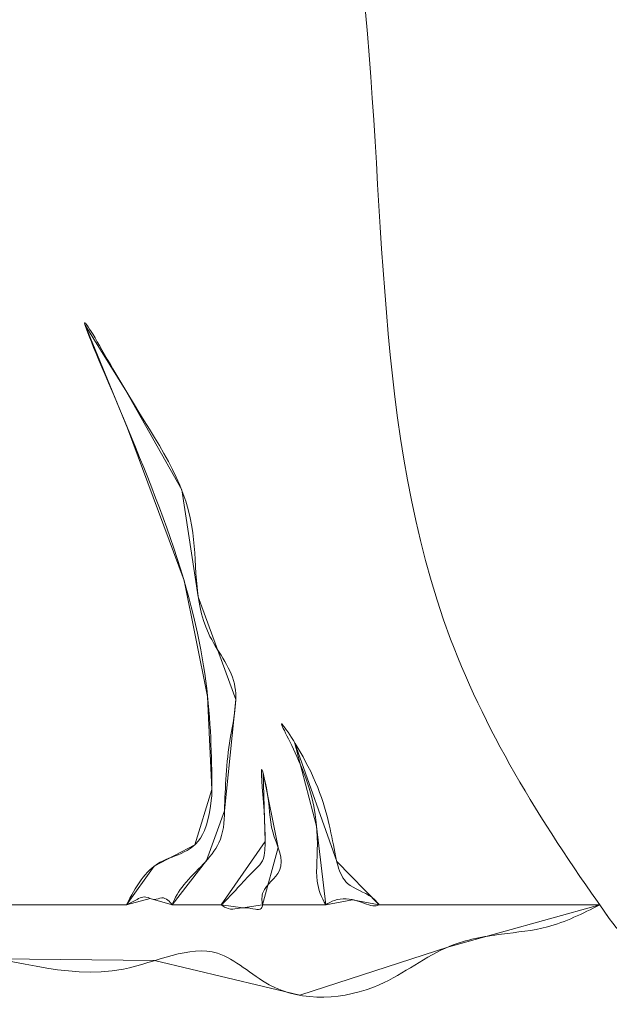
# Model space of a CAD drawing. Units: inches. Extents: x 2083 to 3317, y 1141 to 2115.
# Tile 6 of 256: x 2260 to 2278, y 1296 to 1327. Entities that reach past the tile are written whole.
import ezdxf

# ---------------------------------------------------------------- set-up
doc = ezdxf.new("R2010")
doc.units = ezdxf.units.IN
doc.layers.add('A-FURN', color=8, linetype='Continuous', lineweight=18)
doc.layers.add('www.cadblocksfree.com', color=7, linetype='Continuous', lineweight=9)
doc.layers.add('A-WALL-PATT', color=251, linetype='Continuous', lineweight=13, true_color=0x636466)

# ---------------------------------------------------------------- blocks, each defined once
blk = doc.blocks.new('bed')
at = {"layer": 'www.cadblocksfree.com', "ltscale": 0.2}
for points in [[(3426.379, 1449.413), (3426.379, 1470.154), (3363.387, 1470.154), (3363.387, 1447.076)], [(3363.387, 1445.539), (3363.387, 1443.892)], [(3363.387, 1442.495), (3363.387, 1440.369)], [(3363.387, 1438.564), (3363.387, 1431.137)]]:
    blk.add_lwpolyline(points, dxfattribs=at)
for points, knots in [([(3360.883, 1467.22), (3361.272, 1466.08), (3362.328, 1462.983), (3360.73, 1458.154), (3362.389, 1452.621), (3360.35, 1448.139), (3362.429, 1444.241), (3360.039, 1441.931), (3360.256, 1438.678), (3362.05, 1436.545), (3362.42, 1434.517), (3362.566, 1432.758), (3363.096, 1431.712), (3363.387, 1431.137)], [0, 0, 0, 0, 3.550403, 9.643115, 14.356056, 20.206026, 23.427697, 25.46537, 29.172767, 31.884544, 33.668442, 35.237641, 37.145618, 37.145618, 37.145618, 37.145618]), ([(3367.269, 1444.201), (3369.575, 1444.23), (3373.917, 1444.284), (3385.471, 1449.8), (3379.558, 1446.493), (3376.808, 1444.477), (3372.948, 1444.924), (3370.926, 1443.14), (3368.771, 1443.702), (3367.359, 1443.752), (3366.554, 1443.781)], [0, 0, 0, 0, 8.61026, 16.221274, 18.843057, 23.804898, 27.440828, 29.356102, 31.203478, 33.650687, 33.650687, 33.650687, 33.650687]), ([(3363.387, 1447.076), (3363.429, 1446.99), (3363.529, 1446.784), (3363.731, 1446.461), (3363.506, 1446.154), (3363.665, 1445.905), (3363.559, 1445.673), (3363.444, 1445.584), (3363.387, 1445.539)], [0, 0, 0, 0, 0.293454, 0.701471, 1.003873, 1.254893, 1.47342, 1.69185, 1.69185, 1.69185, 1.69185]), ([(3363.387, 1447.076), (3363.991, 1446.782), (3365.084, 1446.124), (3365.119, 1444.371), (3367.129, 1444.191), (3367.269, 1444.201)], [0.0122268, 0.0122268, 0.0122268, 0.0122268, 0.0594721, 0.1062177, 0.134458, 0.134458, 0.134458, 0.134458]), ([(3366.554, 1443.781), (3366.17, 1443.775), (3365.174, 1443.901), (3364.4, 1444.957), (3363.626, 1445.461), (3363.387, 1445.539)], [0.15648839, 0.15648839, 0.15648839, 0.15648839, 0.18439755, 0.23137648, 0.25059846, 0.25059846, 0.25059846, 0.25059846]), ([(3363.387, 1443.892), (3363.335, 1443.815), (3363.165, 1443.56), (3363.346, 1443.124), (3363.233, 1442.791), (3363.225, 1442.533), (3363.341, 1442.506), (3363.387, 1442.495)], [0, 0, 0, 0, 0.27176, 0.887321, 1.189132, 1.388142, 1.515331, 1.515331, 1.515331, 1.515331]), ([(3363.387, 1443.892), (3363.631, 1443.61), (3364.671, 1442.733), (3364.886, 1442.149), (3369.073, 1442.744), (3366.773, 1442.243), (3365.832, 1442.298), (3364.615, 1441.552), (3363.961, 1442.542), (3363.537, 1442.524), (3363.387, 1442.495)], [0.0595743, 0.0595743, 0.0595743, 0.0595743, 0.0807529, 0.1037415, 0.1697201, 0.1760361, 0.2071372, 0.2404744, 0.2623409, 0.2736605, 0.2736605, 0.2736605, 0.2736605]), ([(3362.928, 1430.813), (3365.944, 1432.958), (3375.455, 1438.993), (3392.12, 1438.03), (3404.249, 1440.73), (3408.408, 1442.961)], [0.102872, 0.102872, 0.102872, 0.102872, 0.37972, 0.957702, 1.313793, 1.313793, 1.313793, 1.313793]), ([(3363.387, 1440.369), (3363.634, 1440.51), (3364.527, 1440.899), (3366.485, 1440.246), (3370.203, 1442.295), (3367.731, 1440.636), (3365.42, 1440.07), (3364.035, 1439.913), (3363.795, 1438.935), (3363.482, 1438.64), (3363.387, 1438.564)], [0.013856, 0.013856, 0.013856, 0.013856, 0.0348738, 0.0888667, 0.1078792, 0.1267378, 0.158714, 0.1937575, 0.2174868, 0.2267221, 0.2267221, 0.2267221, 0.2267221]), ([(3363.387, 1440.369), (3363.445, 1440.274), (3363.571, 1440.065), (3363.607, 1439.678), (3363.531, 1439.31), (3363.405, 1439.003), (3363.329, 1438.751), (3363.372, 1438.611), (3363.387, 1438.564)], [0, 0, 0, 0, 0.329977, 0.725302, 1.129072, 1.442831, 1.734218, 1.878348, 1.878348, 1.878348, 1.878348])]:
    blk.add_open_spline(points, degree=3, knots=knots, dxfattribs=at)

msp = doc.modelspace()

# ---------------------------------------------------------------- hatches: boundary and pattern name
at = {"layer": 'A-WALL-PATT'}
h = msp.add_hatch(color=256, dxfattribs=at)
h.dxf.hatch_style = 1
h.paths.add_polyline_path([(3126.96, 2020.761), (2748.96, 2020.761), (2604.96, 2020.761), (2226.96, 2020.761), (2226.96, 1702.761), (2466.96, 1702.761), (2466.96, 1582.761), (2418.96, 1582.761), (2418.96, 1477.761), (2226.96, 1477.761), (2226.96, 1263.261), (2544.96, 1263.261), (2544.96, 1411.761), (2604.96, 1411.761), (2685.96, 1411.761), (2685.96, 1420.761), (2604.96, 1420.761), (2604.96, 1573.761), (2604.96, 1702.761), (2604.96, 2011.761), (2748.96, 2011.761), (2748.96, 1702.761), (2862.96, 1702.761), (2862.96, 1621.761), (2871.96, 1621.761), (2871.96, 1702.761), (2883.96, 1702.761), (2883.96, 1706.939, -0.026459), (2883.96, 1711.761), (2757.96, 1711.761), (2757.96, 1807.761), (2787.96, 1807.761), (2787.96, 1812.261), (2757.96, 1812.261), (2757.96, 2011.761), (2877.96, 2011.761), (2877.96, 1812.261), (2847.96, 1812.261), (2847.96, 1807.761), (2889.836, 1807.761), (2889.836, 1812.261), (2882.46, 1812.261), (2882.46, 2011.761), (3117.96, 2011.761), (3117.96, 1812.261), (2937.836, 1812.261), (2937.836, 1807.761), (2995.71, 1807.761), (2995.71, 1796.118), (3000.21, 1796.118), (3000.21, 1807.761), (3117.96, 1807.761), (3117.96, 1711.761), (3000.21, 1711.761), (3000.21, 1760.118), (2998.573, 1760.118, -0.020711), (2995.71, 1760.118), (2995.71, 1711.761), (2931.96, 1711.761), (2931.96, 1702.761), (3126.96, 1702.761)])
h.paths.add_polyline_path([(2471.46, 2011.761), (2471.46, 1810.011), (2462.717, 1810.011), (2462.717, 1805.511), (2505.96, 1805.511), (2505.96, 1810.011), (2475.96, 1810.011), (2475.96, 2011.761), (2595.96, 2011.761), (2595.96, 1810.011), (2565.96, 1810.011), (2565.96, 1805.511), (2595.96, 1805.511), (2595.96, 1711.761), (2235.96, 1711.761), (2235.96, 1805.511), (2353.71, 1805.511), (2353.71, 1796.054), (2358.21, 1796.054), (2358.21, 1805.511), (2414.717, 1805.511), (2414.717, 1810.011), (2235.96, 1810.011), (2235.96, 2011.761)], flags=16)
h.paths.add_polyline_path([(2270.205, 1994.61), (2270.205, 1970.61), (2246.205, 1970.61), (2246.205, 1994.61)], flags=0)
edge = h.paths.add_edge_path(flags=0)
edge.add_ellipse((2332.027, 1899.798), major_axis=(-3.043, 3.043), ratio=0.168252, start_angle=-161.3322, end_angle=-156.3071, ccw=False)
edge.add_ellipse((2333.082, 1898.744), major_axis=(-1.055, 1.055), ratio=0.453532, start_angle=-123.371, end_angle=-94.1591)
edge = h.paths.add_edge_path(flags=0)
edge.add_ellipse((2332.027, 1968.876), major_axis=(3.043, 3.043), ratio=0.168252, start_angle=18.6678, end_angle=23.6929)
edge.add_spline(control_points=[(2332.926, 1970.691), (2332.227, 1970.336), (2330.894, 1969.659), (2328.413, 1970.932), (2327.204, 1967.749), (2324.71, 1969.956), (2322.533, 1967.012), (2320.013, 1971.296), (2317.68, 1968.158), (2316.041, 1967.102), (2315.427, 1966.81)], knot_values=[0, 0, 0, 0, 2.267059, 4.324559, 6.685584, 8.878641, 11.121502, 14.300359, 17.755284, 19.732645, 19.732645, 19.732645, 19.732645], degree=3, periodic=0)
edge.add_ellipse((2332.027, 1968.876), major_axis=(3.043, 3.043), ratio=0.168252, start_angle=18.6678, end_angle=23.6929, ccw=False)
edge.add_ellipse((2333.082, 1969.931), major_axis=(1.055, 1.055), ratio=0.453532, start_angle=56.629, end_angle=85.8409, ccw=False)
edge = h.paths.add_edge_path(flags=0)
edge.add_spline(control_points=[(2296.428, 1967.988), (2293.628, 1965.336), (2287.704, 1959.727), (2299.744, 1949.996), (2294.533, 1935.669), (2290.573, 1920.604), (2293.394, 1909.974), (2296.185, 1904.967)], knot_values=[0.099185, 0.099185, 0.099185, 0.099185, 0.345301, 0.619822, 0.982653, 1.386093, 1.810555, 1.810555, 1.810555, 1.810555], degree=3, periodic=0)
edge.add_spline(control_points=[(2296.185, 1904.967), (2297.384, 1902.619), (2298.001, 1901.949), (2298.553, 1901.468)], knot_values=[0.006246, 0.006246, 0.006246, 0.006246, 0.055476, 0.055476, 0.055476, 0.055476], degree=3, periodic=0)
edge.add_spline(control_points=[(2298.553, 1901.468), (2297.259, 1900.923), (2295.225, 1900.232), (2293.06, 1900.614), (2292.101, 1900.788), (2292.09, 1900.791)], knot_values=[0.312835, 0.312835, 0.312835, 0.312835, 0.40178, 0.474987, 0.475903, 0.475903, 0.475903, 0.475903], degree=3, periodic=0)
edge.add_arc((2292.794, 1904.664), 3.937, 215.4209, 259.6982, ccw=False)
edge.add_spline(control_points=[(2289.585, 1902.382), (2289.477, 1902.535), (2289.368, 1902.688), (2289.261, 1902.841)], knot_values=[0.102872, 0.102872, 0.102872, 0.102872, 0.116896, 0.116896, 0.116896, 0.116896], degree=3, periodic=0)
edge.add_spline(control_points=[(2289.261, 1902.841), (2288.687, 1902.55), (2287.64, 1902.02), (2285.881, 1901.874), (2283.853, 1901.504), (2281.72, 1899.711), (2278.467, 1899.493), (2276.157, 1901.883), (2272.259, 1899.804), (2267.778, 1901.843), (2262.244, 1900.184), (2257.415, 1901.782), (2254.318, 1900.726), (2253.178, 1900.337)], knot_values=[0, 0, 0, 0, 1.907977, 3.477176, 5.261074, 7.972851, 11.680248, 13.717921, 16.939592, 22.789562, 27.502503, 33.595215, 37.145618, 37.145618, 37.145618, 37.145618], degree=3, periodic=0)
edge.add_line((2253.178, 1900.337), (2250.244, 1902.841))
edge.add_line((2250.244, 1902.841), (2250.244, 1965.833))
edge.add_line((2250.244, 1965.833), (2253.178, 1968.337))
edge.add_spline(control_points=[(2253.178, 1968.337), (2254.318, 1967.948), (2257.415, 1966.892), (2262.244, 1968.49), (2267.778, 1966.831), (2271.527, 1968.537), (2273.876, 1967.828), (2274.207, 1967.728)], knot_values=[0, 0, 0, 0, 0.09018, 0.244935, 0.364644, 0.513233, 0.537855, 0.537855, 0.537855, 0.537855], degree=3, periodic=0)
edge.add_arc((2274.353, 1963.793), 3.937, 72.0511, 92.1279, ccw=False)
edge.add_arc((2281.297, 1985.23), 18.596, 252.0511, 288.5657)
edge.add_arc((2292.317, 1956.029), 12.646, 71.0268, 113.7782, ccw=False)
edge = h.paths.add_edge_path(flags=0)
edge.add_spline(control_points=[(2274.899, 1951.856), (2275.066, 1951.617), (2275.233, 1951.377), (2275.398, 1951.136)], knot_values=[1.409916, 1.409916, 1.409916, 1.409916, 1.43159, 1.43159, 1.43159, 1.43159], degree=3, periodic=0)
edge.add_spline(control_points=[(2275.398, 1951.136), (2275.792, 1950.562), (2276.179, 1949.984), (2276.546, 1949.397)], knot_values=[1.358238, 1.358238, 1.358238, 1.358238, 1.409916, 1.409916, 1.409916, 1.409916], degree=3, periodic=0)
edge.add_line((2276.546, 1949.397), (2277.437, 1947.862))
edge.add_spline(control_points=[(2277.437, 1947.862), (2276.304, 1945.673), (2274.64, 1942.427), (2274.632, 1938.094), (2272.799, 1930.852), (2274.356, 1943.897), (2275.948, 1947.923), (2276.546, 1949.397)], knot_values=[0.005632, 0.005632, 0.005632, 0.005632, 0.186014, 0.266002, 0.357087, 0.59639, 0.739732, 0.739732, 0.739732, 0.739732], degree=3, periodic=0)
edge.add_spline(control_points=[(2276.546, 1949.397), (2276.179, 1949.984), (2275.792, 1950.562), (2275.398, 1951.136)], knot_values=[1.358238, 1.358238, 1.358238, 1.358238, 1.409916, 1.409916, 1.409916, 1.409916], degree=3, periodic=0)
edge.add_spline(control_points=[(2275.398, 1951.136), (2274.943, 1950.08), (2274.208, 1948.025), (2273.935, 1944.851), (2272.469, 1937.627), (2273.466, 1945.696), (2274.701, 1951.059), (2274.899, 1951.856)], knot_values=[0.104364, 0.104364, 0.104364, 0.104364, 0.189636, 0.269624, 0.36071, 0.600013, 0.644622, 0.644622, 0.644622, 0.644622], degree=3, periodic=0)
h.paths.add_polyline_path([(2269.168, 1963.128, -0.357527), (2268.171, 1960.976, -0.092561), (2268.171, 1939.436, -0.357527), (2269.168, 1937.285, -0.357527), (2267.016, 1938.282, -0.164785), (2254.686, 1938.282, -0.357527), (2252.534, 1937.285, -0.357527), (2253.531, 1939.436, -0.092561), (2253.531, 1960.976, -0.357527), (2252.534, 1963.128, -0.357527), (2254.686, 1962.131, -0.164785), (2267.016, 1962.131, -0.357527)], flags=0)
h.paths.add_polyline_path([(2248.874, 1967.802), (2248.874, 1957.028), (2249.458, 1957.028), (2249.458, 1911.647), (2248.874, 1911.647), (2248.874, 1900.873), (2246.512, 1900.873, 0.197327), (2244.15, 1902.457), (2244.15, 1966.218, 0.197327), (2246.512, 1967.802)], flags=0)
h.paths.add_polyline_path([(2269.168, 1931.389, -0.357527), (2268.171, 1929.238, -0.092561), (2268.171, 1907.698, -0.357527), (2269.168, 1905.547, -0.357527), (2267.016, 1906.544, -0.164785), (2254.686, 1906.544, -0.357527), (2252.534, 1905.547, -0.357527), (2253.531, 1907.698, -0.092561), (2253.531, 1929.238, -0.357527), (2252.534, 1931.389, -0.357527), (2254.686, 1930.392, -0.164785), (2267.016, 1930.392, -0.357527)], flags=0)
edge = h.paths.add_edge_path(flags=0)
edge.add_spline(control_points=[(2276.197, 1906.724), (2276.168, 1909.029), (2276.114, 1913.372), (2270.598, 1924.925), (2273.905, 1919.013), (2275.922, 1916.262), (2275.475, 1912.402), (2277.258, 1910.381), (2276.696, 1908.225), (2276.646, 1906.813), (2276.618, 1906.008)], knot_values=[0, 0, 0, 0, 8.61026, 16.221274, 18.843057, 23.804898, 27.440828, 29.356102, 31.203478, 33.650687, 33.650687, 33.650687, 33.650687], degree=3, periodic=0)
edge.add_spline(control_points=[(2276.618, 1906.008), (2276.623, 1905.624), (2276.498, 1904.629), (2275.442, 1903.855), (2274.937, 1903.08), (2274.859, 1902.841)], knot_values=[0.156488, 0.156488, 0.156488, 0.156488, 0.184398, 0.231376, 0.250598, 0.250598, 0.250598, 0.250598], degree=3, periodic=0)
edge.add_line((2274.859, 1902.841), (2276.506, 1902.841))
edge.add_spline(control_points=[(2276.506, 1902.841), (2276.788, 1903.085), (2277.665, 1904.125), (2278.25, 1904.341), (2277.654, 1908.527), (2278.156, 1906.228), (2278.1, 1905.286), (2278.847, 1904.069), (2277.857, 1903.415), (2277.874, 1902.991), (2277.904, 1902.841)], knot_values=[0.059574, 0.059574, 0.059574, 0.059574, 0.080753, 0.103741, 0.16972, 0.176036, 0.207137, 0.240474, 0.262341, 0.27366, 0.27366, 0.27366, 0.27366], degree=3, periodic=0)
edge.add_line((2277.904, 1902.841), (2280.03, 1902.841))
edge.add_spline(control_points=[(2280.03, 1902.841), (2279.888, 1903.088), (2279.499, 1903.982), (2280.152, 1905.939), (2278.104, 1909.658), (2279.762, 1907.185), (2280.328, 1904.875), (2280.485, 1903.49), (2281.463, 1903.249), (2281.758, 1902.936), (2281.834, 1902.841)], knot_values=[0.013856, 0.013856, 0.013856, 0.013856, 0.034874, 0.088867, 0.107879, 0.126738, 0.158714, 0.193757, 0.217487, 0.226722, 0.226722, 0.226722, 0.226722], degree=3, periodic=0)
edge.add_spline(control_points=[(2281.834, 1902.841), (2281.788, 1902.827), (2281.647, 1902.783), (2281.396, 1902.859), (2281.088, 1902.985), (2280.721, 1903.061), (2280.333, 1903.026), (2280.125, 1902.899), (2280.03, 1902.841)], knot_values=[0, 0, 0, 0, 0.14413, 0.435517, 0.749276, 1.153046, 1.548371, 1.878348, 1.878348, 1.878348, 1.878348], degree=3, periodic=0)
edge.add_line((2280.03, 1902.841), (2277.904, 1902.841))
edge.add_spline(control_points=[(2277.904, 1902.841), (2277.893, 1902.796), (2277.865, 1902.68), (2277.607, 1902.687), (2277.274, 1902.801), (2276.838, 1902.62), (2276.584, 1902.789), (2276.506, 1902.841)], knot_values=[0, 0, 0, 0, 0.127189, 0.326199, 0.628009, 1.24357, 1.515331, 1.515331, 1.515331, 1.515331], degree=3, periodic=0)
edge.add_line((2276.506, 1902.841), (2274.859, 1902.841))
edge.add_spline(control_points=[(2274.859, 1902.841), (2274.814, 1902.899), (2274.725, 1903.013), (2274.493, 1903.119), (2274.244, 1902.961), (2273.937, 1903.185), (2273.614, 1902.983), (2273.408, 1902.883), (2273.322, 1902.841)], knot_values=[0, 0, 0, 0, 0.21843, 0.436957, 0.687977, 0.990379, 1.398396, 1.69185, 1.69185, 1.69185, 1.69185], degree=3, periodic=0)
edge.add_spline(control_points=[(2273.322, 1902.841), (2273.617, 1903.446), (2274.274, 1904.538), (2276.027, 1904.574), (2276.207, 1906.584), (2276.197, 1906.724)], knot_values=[0.012227, 0.012227, 0.012227, 0.012227, 0.059472, 0.106218, 0.134458, 0.134458, 0.134458, 0.134458], degree=3, periodic=0)
h.paths.add_polyline_path([(2270.776, 1897.79), (2270.776, 1873.79), (2246.776, 1873.79), (2246.776, 1897.79)], flags=0)
h.paths.add_polyline_path([(2353.71, 1760.005), (2353.71, 1760.054), (2358.21, 1760.054, -0.033729)], flags=0)
h.paths.add_polyline_path([(2321.819, 1737.529), (2341.995, 1737.529, -0.414214), (2343.203, 1736.321), (2343.203, 1721.021, -0.414214), (2341.995, 1719.813), (2321.819, 1719.813, -0.414214), (2320.611, 1721.021), (2320.611, 1736.321, -0.414214)], flags=0)
h.paths.add_polyline_path([(2324.235, 1736.321), (2339.579, 1736.321, -0.414214), (2341.995, 1733.905), (2341.995, 1725.45, -0.414214), (2339.579, 1723.034), (2333.681, 1723.034), (2333.845, 1722.045, -0.870646), (2335.425, 1721.826, -0.767327), (2333.923, 1721.423), (2331.291, 1721.423, -0.767327), (2329.788, 1721.826, -0.870646), (2331.368, 1722.045), (2331.533, 1723.034), (2324.235, 1723.034, -0.414214), (2321.819, 1725.45), (2321.819, 1733.905, -0.414214)], flags=0)
h.paths.add_polyline_path([(2570.484, 1928.615), (2589.684, 1928.615), (2590.169, 1928.615), (2590.169, 1904.993), (2570.484, 1904.993)], flags=0)
h.paths.add_polyline_path([(2574.447, 1927.264, -1), (2572.829, 1927.264, -1)], flags=0)
h.paths.add_polyline_path([(2573.09, 1926.941), (2573.925, 1927.776), (2574.148, 1927.553), (2573.313, 1926.718)], flags=0)
h.paths.add_polyline_path([(2578.779, 1919.73, -1), (2571.592, 1919.73, -1)], flags=0)
h.paths.add_polyline_path([(2578.385, 1919.73, -1), (2571.985, 1919.73, -1)], flags=0)
h.paths.add_polyline_path([(2331.596, 1729.476, -1), (2333.618, 1729.476, -1)], flags=0)
h.paths.add_polyline_path([(2578.034, 1927.264, -1), (2576.416, 1927.264, -1)], flags=0)
h.paths.add_polyline_path([(2576.689, 1927.531), (2576.912, 1927.754), (2577.747, 1926.919), (2577.524, 1926.696)], flags=0)
h.paths.add_polyline_path([(2578.139, 1909.86, -1), (2572.232, 1909.86, -1)], flags=0)
h.paths.add_polyline_path([(2577.745, 1909.86, -1), (2572.625, 1909.86, -1)], flags=0)
h.paths.add_polyline_path([(2583.798, 1927.264, -1), (2582.179, 1927.264, -1)], flags=0)
h.paths.add_polyline_path([(2582.719, 1927.754), (2583.554, 1926.919), (2583.331, 1926.696), (2582.496, 1927.531)], flags=0)
h.paths.add_polyline_path([(2582.496, 1927.531), (2582.719, 1927.754), (2583.554, 1926.919), (2583.331, 1926.696)], flags=0)
h.paths.add_polyline_path([(2587.739, 1920.53, -1), (2581.832, 1920.53, -1)], flags=0)
h.paths.add_polyline_path([(2587.345, 1920.53, -1), (2582.225, 1920.53, -1)], flags=0)
h.paths.add_polyline_path([(2587.385, 1927.264, -1), (2585.766, 1927.264, -1)], flags=0)
h.paths.add_polyline_path([(2586.082, 1926.98), (2586.917, 1927.815), (2587.14, 1927.593), (2586.305, 1926.758)], flags=0)
h.paths.add_polyline_path([(2588.379, 1910.66, -1), (2581.192, 1910.66, -1)], flags=0)
h.paths.add_polyline_path([(2587.985, 1910.66, -1), (2581.585, 1910.66, -1)], flags=0)
h.paths.add_polyline_path([(2417.168, 1729.478), (2437.344, 1729.478, -0.414214), (2438.552, 1728.27), (2438.552, 1712.969, -0.414214), (2437.344, 1711.761), (2417.168, 1711.761, -0.414214), (2415.96, 1712.969), (2415.96, 1728.27, -0.414214)], flags=0)
h.paths.add_polyline_path([(2419.584, 1728.27), (2434.928, 1728.27, -0.414214), (2437.344, 1725.854), (2437.344, 1717.398, -0.414214), (2434.928, 1714.983), (2429.029, 1714.983), (2429.194, 1713.994, -0.870646), (2430.774, 1713.775, -0.767327), (2429.271, 1713.372), (2426.64, 1713.372, -0.767327), (2425.137, 1713.775, -0.870646), (2426.717, 1713.994), (2426.882, 1714.983), (2419.584, 1714.983, -0.414214), (2417.168, 1717.398), (2417.168, 1725.854, -0.414214)], flags=0)
h.paths.add_polyline_path([(2419.584, 1728.27), (2434.928, 1728.27, -0.414214), (2437.344, 1725.854), (2437.344, 1717.398, -0.414214), (2434.928, 1714.983), (2429.029, 1714.983), (2428.358, 1719.009), (2427.553, 1719.009), (2426.882, 1714.983), (2419.584, 1714.983, -0.414214), (2417.168, 1717.398), (2417.168, 1725.854, -0.414214)], flags=0)
h.paths.add_polyline_path([(2426.944, 1721.425, -1), (2428.967, 1721.425, -1)], flags=0)
h.paths.add_polyline_path([(2475.96, 1702.761), (2595.96, 1702.761), (2595.96, 1582.761), (2475.96, 1582.761)], flags=16)
h.paths.add_polyline_path([(2427.96, 1573.761), (2595.96, 1573.761), (2595.96, 1468.761), (2595.96, 1420.761), (2384.46, 1420.761), (2384.46, 1468.761), (2427.96, 1468.761)], flags=16)
h.paths.add_polyline_path([(2379.96, 1468.761), (2379.96, 1420.761), (2235.96, 1420.761), (2235.96, 1468.761)], flags=16)
h.paths.add_polyline_path([(2317.816, 1466.696), (2337.992, 1466.696, -0.414214), (2339.2, 1465.488), (2339.2, 1450.187, -0.414214), (2337.992, 1448.979), (2317.816, 1448.979, -0.414214), (2316.608, 1450.187), (2316.608, 1465.488, -0.414214)], flags=0)
h.paths.add_polyline_path([(2320.232, 1465.488), (2335.576, 1465.488, -0.414214), (2337.992, 1463.072), (2337.992, 1454.616, -0.414214), (2335.576, 1452.2), (2329.677, 1452.2), (2329.842, 1451.212, -0.870646), (2331.422, 1450.992, -0.767327), (2329.92, 1450.59), (2327.288, 1450.59, -0.767327), (2325.785, 1450.992, -0.870646), (2327.365, 1451.212), (2327.53, 1452.2), (2320.232, 1452.2, -0.414214), (2317.816, 1454.616), (2317.816, 1463.072, -0.414214)], flags=0)
h.paths.add_polyline_path([(2320.232, 1465.488), (2335.576, 1465.488, -0.414214), (2337.992, 1463.072), (2337.992, 1454.616, -0.414214), (2335.576, 1452.2), (2329.677, 1452.2), (2329.006, 1456.227), (2328.201, 1456.227), (2327.53, 1452.2), (2320.232, 1452.2, -0.414214), (2317.816, 1454.616), (2317.816, 1463.072, -0.414214)], flags=0)
h.paths.add_polyline_path([(2327.593, 1458.643, -1), (2329.615, 1458.643, -1)], flags=0)
h.paths.add_polyline_path([(2244.412, 1433.34), (2241.921, 1433.34, -0.414214), (2240.018, 1435.244), (2240.018, 1440.953, -0.414211), (2241.921, 1442.856), (2244.412, 1442.856, -1.976472)], flags=0)
h.paths.add_polyline_path([(2245.357, 1434.398, -0.414214), (2245.357, 1441.799, -2.144098)], flags=0)
h.paths.add_polyline_path([(2535.96, 1416.261), (2535.96, 1272.261), (2235.96, 1272.261), (2235.96, 1416.261)], flags=16)
h.paths.add_polyline_path([(2260.12, 1384.293), (2260.12, 1362.039), (2237.865, 1362.039), (2237.865, 1384.293)], flags=0)
edge = h.paths.add_edge_path(flags=0)
edge.add_line((2318.252, 1362.093), (2318.146, 1362.001))
edge.add_ellipse((2317.445, 1360.431), major_axis=(2.822, 2.822), ratio=0.168252, start_angle=18.6678, end_angle=20.9481, ccw=False)
edge.add_ellipse((2318.423, 1361.409), major_axis=(0.978, 0.978), ratio=0.453532, start_angle=56.629, end_angle=70.2262, ccw=False)
edge = h.paths.add_edge_path(flags=0)
edge.add_line((2319.107, 1295.571), (2319.015, 1295.677))
edge.add_ellipse((2317.445, 1296.378), major_axis=(-2.822, 2.822), ratio=0.168252, start_angle=-161.3322, end_angle=-159.0519, ccw=False)
edge.add_ellipse((2318.423, 1295.4), major_axis=(-0.978, 0.978), ratio=0.453532, start_angle=-123.371, end_angle=-109.7738)
edge = h.paths.add_edge_path(flags=0)
edge.add_spline(control_points=[(2284.21, 1301.17), (2284.581, 1300.445), (2284.891, 1299.892), (2285.16, 1299.461)], knot_values=[0.039066, 0.039066, 0.039066, 0.039066, 0.055476, 0.055476, 0.055476, 0.055476], degree=3, periodic=0)
edge.add_line((2285.16, 1299.461), (2284.21, 1301.17))
edge = h.paths.add_edge_path(flags=0)
edge.add_line((2280.412, 1297.298), (2283.37, 1297.036))
edge.add_line((2283.37, 1297.036), (2286.406, 1297.926))
edge.add_spline(control_points=[(2286.406, 1297.926), (2285.305, 1297.463), (2284.345, 1297.129), (2283.37, 1297.036)], knot_values=[0.394369, 0.394369, 0.394369, 0.394369, 0.475903, 0.475903, 0.475903, 0.475903], degree=3, periodic=0)
edge.add_spline(control_points=[(2283.37, 1297.036), (2283.281, 1297.028), (2282.316, 1296.957), (2281.313, 1297.134), (2280.423, 1297.296), (2280.412, 1297.298)], knot_values=[0.312835, 0.312835, 0.312835, 0.312835, 0.320246, 0.393453, 0.394369, 0.394369, 0.394369, 0.394369], degree=3, periodic=0)
edge = h.paths.add_edge_path(flags=0)
edge.add_line((2284.436, 1359.607), (2280.446, 1355.328))
edge.add_line((2280.446, 1355.328), (2279.58, 1351.018))
edge.add_line((2279.58, 1351.018), (2282.413, 1346.58))
edge.add_spline(control_points=[(2282.413, 1346.58), (2283.153, 1345.589), (2284.253, 1344.029), (2284.801, 1342.387), (2284.935, 1341.806)], knot_values=[1.240098, 1.240098, 1.240098, 1.240098, 1.332892, 1.382712, 1.382712, 1.382712, 1.382712], degree=3, periodic=0)
edge.add_spline(control_points=[(2284.935, 1341.806), (2285.319, 1340.141), (2285.233, 1338.409), (2284.91, 1336.654)], knot_values=[1.097484, 1.097484, 1.097484, 1.097484, 1.240098, 1.240098, 1.240098, 1.240098], degree=3, periodic=0)
edge.add_spline(control_points=[(2284.91, 1336.654), (2284.587, 1334.899), (2284.027, 1333.12), (2283.463, 1331.361)], knot_values=[0.95487, 0.95487, 0.95487, 0.95487, 1.097484, 1.097484, 1.097484, 1.097484], degree=3, periodic=0)
edge.add_line((2283.463, 1331.361), (2281.89, 1326.153))
edge.add_line((2281.89, 1326.153), (2280.756, 1321.056))
edge.add_line((2280.756, 1321.056), (2280.299, 1316.002))
edge.add_line((2280.299, 1316.002), (2280.716, 1310.95))
edge.add_line((2280.716, 1310.95), (2282.028, 1305.972))
edge.add_line((2282.028, 1305.972), (2284.21, 1301.17))
edge.add_spline(control_points=[(2284.21, 1301.17), (2283.341, 1302.73), (2282.612, 1304.336), (2282.028, 1305.972)], knot_values=[0.099185, 0.099185, 0.099185, 0.099185, 0.241799, 0.241799, 0.241799, 0.241799], degree=3, periodic=0)
edge.add_spline(control_points=[(2282.028, 1305.972), (2281.444, 1307.608), (2281.005, 1309.273), (2280.716, 1310.95)], knot_values=[0.241799, 0.241799, 0.241799, 0.241799, 0.384413, 0.384413, 0.384413, 0.384413], degree=3, periodic=0)
edge.add_spline(control_points=[(2280.716, 1310.95), (2280.433, 1312.588), (2280.289, 1314.277), (2280.299, 1315.962), (2280.299, 1316.002)], knot_values=[0.384413, 0.384413, 0.384413, 0.384413, 0.523647, 0.527028, 0.527028, 0.527028, 0.527028], degree=3, periodic=0)
edge.add_spline(control_points=[(2280.299, 1316.002), (2280.312, 1317.687), (2280.478, 1319.368), (2280.756, 1321.056)], knot_values=[0.527028, 0.527028, 0.527028, 0.527028, 0.669642, 0.669642, 0.669642, 0.669642], degree=3, periodic=0)
edge.add_spline(control_points=[(2280.756, 1321.056), (2281.035, 1322.744), (2281.426, 1324.44), (2281.89, 1326.153)], knot_values=[0.669642, 0.669642, 0.669642, 0.669642, 0.812256, 0.812256, 0.812256, 0.812256], degree=3, periodic=0)
edge.add_spline(control_points=[(2281.89, 1326.153), (2282.264, 1327.533), (2282.788, 1329.262), (2283.353, 1331.018), (2283.463, 1331.361)], knot_values=[0.812256, 0.812256, 0.812256, 0.812256, 0.927087, 0.95487, 0.95487, 0.95487, 0.95487], degree=3, periodic=0)
edge.add_line((2283.463, 1331.361), (2284.91, 1336.654))
edge.add_line((2284.91, 1336.654), (2284.935, 1341.806))
edge.add_line((2284.935, 1341.806), (2282.413, 1346.58))
edge.add_spline(control_points=[(2282.413, 1346.58), (2281.275, 1348.104), (2280.078, 1349.57), (2279.58, 1351.018)], knot_values=[1.382712, 1.382712, 1.382712, 1.382712, 1.525326, 1.525326, 1.525326, 1.525326], degree=3, periodic=0)
edge.add_spline(control_points=[(2279.58, 1351.018), (2279.443, 1351.415), (2279.136, 1352.857), (2279.735, 1354.29), (2280.446, 1355.328)], knot_values=[1.525326, 1.525326, 1.525326, 1.525326, 1.564439, 1.667941, 1.667941, 1.667941, 1.667941], degree=3, periodic=0)
edge.add_spline(control_points=[(2280.446, 1355.328), (2281.426, 1356.758), (2282.931, 1358.183), (2284.436, 1359.607)], knot_values=[1.667941, 1.667941, 1.667941, 1.667941, 1.810555, 1.810555, 1.810555, 1.810555], degree=3, periodic=0)
edge.add_arc((2280.623, 1348.518), 11.726, 71.0268, 113.7782)
edge.add_arc((2270.405, 1375.595), 17.244, 252.0511, 288.5657, ccw=False)
edge.add_arc((2263.966, 1355.718), 3.651, 72.0511, 92.1279)
edge.add_arc((2263.966, 1355.718), 3.651, 92.1279, 177.9851)
edge.add_spline(control_points=[(2260.318, 1355.846), (2260.26, 1354.221), (2260.551, 1350.187), (2262.999, 1346.766), (2264.473, 1344.649)], knot_values=[1.43159, 1.43159, 1.43159, 1.43159, 1.564144, 1.770695, 1.770695, 1.770695, 1.770695], degree=3, periodic=0)
edge.add_line((2264.473, 1344.649), (2264.936, 1343.983))
edge.add_spline(control_points=[(2263.801, 1340.248), (2263.843, 1340.514), (2264.067, 1341.756), (2264.513, 1343.002), (2264.935, 1343.981)], knot_values=[0.53657, 0.53657, 0.53657, 0.53657, 0.559349, 0.644622, 0.644622, 0.644622, 0.644622], degree=3, periodic=0)
edge.add_spline(control_points=[(2264.935, 1343.981), (2265.118, 1343.715), (2265.299, 1343.448), (2265.477, 1343.179)], knot_values=[1.384077, 1.384077, 1.384077, 1.384077, 1.409916, 1.409916, 1.409916, 1.409916], degree=3, periodic=0)
edge.add_spline(control_points=[(2265.477, 1343.179), (2265.655, 1342.911), (2265.829, 1342.641), (2265.999, 1342.369)], knot_values=[1.358238, 1.358238, 1.358238, 1.358238, 1.384077, 1.384077, 1.384077, 1.384077], degree=3, periodic=0)
edge.add_line((2265.999, 1342.369), (2266.826, 1340.946))
edge.add_spline(control_points=[(2266.826, 1340.946), (2268.894, 1337.09), (2271.398, 1325.843), (2270.516, 1310.569), (2275.919, 1301.861), (2277.79, 1299.199)], knot_values=[0.116896, 0.116896, 0.116896, 0.116896, 0.472987, 1.050969, 1.313793, 1.313793, 1.313793, 1.313793], degree=3, periodic=0)
edge.add_spline(control_points=[(2277.79, 1299.199), (2277.839, 1299.128), (2277.889, 1299.057), (2277.94, 1298.987)], knot_values=[0.109884, 0.109884, 0.109884, 0.109884, 0.116896, 0.116896, 0.116896, 0.116896], degree=3, periodic=0)
edge.add_line((2277.94, 1298.987), (2277.789, 1299.199))
edge.add_spline(control_points=[(2277.789, 1299.199), (2277.257, 1298.929), (2276.286, 1298.438), (2275.039, 1298.334), (2274.383, 1298.239), (2274.215, 1298.209)], knot_values=[33.12187, 33.12187, 33.12187, 33.12187, 35.029056, 36.598255, 37.144827, 37.144827, 37.144827, 37.144827], degree=3, periodic=0)
edge.add_line((2274.215, 1298.209), (2273.073, 1297.893))
edge.add_spline(control_points=[(2273.073, 1297.893), (2272.323, 1297.58), (2271.039, 1296.511), (2269.248, 1296.226), (2268.423, 1296.375)], knot_values=[26.532584, 26.532584, 26.532584, 26.532584, 29.198919, 31.839101, 31.839101, 31.839101, 31.839101], degree=3, periodic=0)
edge.add_line((2268.423, 1296.375), (2263.879, 1297.458))
edge.add_spline(control_points=[(2263.879, 1297.458), (2263.556, 1297.359), (2261.86, 1296.839), (2260.239, 1297.282), (2258.933, 1297.516)], knot_values=[15.919551, 15.919551, 15.919551, 15.919551, 16.939592, 21.226067, 21.226067, 21.226067, 21.226067], degree=3, periodic=0)
edge.add_line((2258.933, 1297.516), (2254.055, 1297.329))
edge.add_spline(control_points=[(2254.055, 1297.329), (2253.756, 1297.296), (2252.114, 1297.165), (2250.462, 1297.544), (2249.13, 1297.668)], knot_values=[5.306517, 5.306517, 5.306517, 5.306517, 6.276435, 10.613034, 10.613034, 10.613034, 10.613034], degree=3, periodic=0)
edge.add_line((2249.13, 1297.668), (2244.332, 1296.878))
edge.add_line((2244.332, 1296.878), (2241.611, 1299.199))
edge.add_line((2241.611, 1299.199), (2241.611, 1357.609))
edge.add_line((2241.611, 1357.609), (2244.332, 1359.931))
edge.add_line((2244.332, 1359.931), (2252.729, 1359.543))
edge.add_spline(control_points=[(2252.729, 1359.543), (2252.871, 1359.546), (2253.306, 1359.548), (2253.74, 1359.514), (2254.032, 1359.482)], knot_values=[0.233291, 0.233291, 0.233291, 0.233291, 0.244935, 0.268927, 0.268927, 0.268927, 0.268927], degree=3, periodic=0)
edge.add_line((2254.032, 1359.482), (2259.587, 1359.416))
edge.add_spline(control_points=[(2259.587, 1359.416), (2260.677, 1359.629), (2262.073, 1359.897), (2263.524, 1359.459), (2263.83, 1359.366)], knot_values=[0.422516, 0.422516, 0.422516, 0.422516, 0.513233, 0.537855, 0.537855, 0.537855, 0.537855], degree=3, periodic=0)
edge.add_arc((2263.966, 1355.718), 3.651, 72.0511, 92.1279, ccw=False)
edge.add_arc((2270.405, 1375.595), 17.244, 252.0511, 288.5657)
edge.add_arc((2280.623, 1348.518), 11.726, 71.0268, 113.7782, ccw=False)
h.paths.add_polyline_path([(2240.341, 1359.435), (2240.341, 1349.444), (2240.882, 1349.444), (2240.882, 1307.365), (2240.341, 1307.365), (2240.341, 1297.374), (2238.15, 1297.374, 0.197327), (2235.96, 1298.843), (2235.96, 1357.966, 0.197327), (2238.15, 1359.435)], flags=0)
h.paths.add_polyline_path([(2259.158, 1355.101, -0.357527), (2258.233, 1353.106, -0.092561), (2258.233, 1333.133, -0.357527), (2259.158, 1331.138, -0.357527), (2257.163, 1332.062, -0.164785), (2245.729, 1332.062, -0.357527), (2243.735, 1331.138, -0.357527), (2244.659, 1333.133, -0.092561), (2244.659, 1353.106, -0.357527), (2243.735, 1355.101, -0.357527), (2245.729, 1354.176, -0.164785), (2257.163, 1354.176, -0.357527)], flags=0)
edge = h.paths.add_edge_path(flags=0)
edge.add_line((2265.999, 1342.369), (2266.826, 1340.946))
edge.add_line((2266.826, 1340.946), (2265.308, 1337.814))
edge.add_line((2265.308, 1337.814), (2264.358, 1334.653))
edge.add_line((2264.358, 1334.653), (2264.262, 1333.8))
edge.add_spline(control_points=[(2264.262, 1333.8), (2264.208, 1333.187), (2264.162, 1332.366), (2264.007, 1331.414), (2263.969, 1331.202)], knot_values=[0.464444, 0.464444, 0.464444, 0.464444, 0.516691, 0.531608, 0.531608, 0.531608, 0.531608], degree=3, periodic=0)
edge.add_spline(control_points=[(2263.969, 1331.202), (2263.775, 1330.119), (2263.424, 1328.791), (2263.257, 1328.531), (2263.234, 1328.515)], knot_values=[0.372682, 0.372682, 0.372682, 0.372682, 0.44885, 0.464444, 0.464444, 0.464444, 0.464444], degree=3, periodic=0)
edge.add_spline(control_points=[(2263.234, 1328.515), (2263.096, 1328.42), (2263.131, 1329.301), (2263.275, 1330.616)], knot_values=[0.280919, 0.280919, 0.280919, 0.280919, 0.372682, 0.372682, 0.372682, 0.372682], degree=3, periodic=0)
edge.add_spline(control_points=[(2263.275, 1330.616), (2263.419, 1331.93), (2263.672, 1333.677), (2263.97, 1335.315)], knot_values=[0.189157, 0.189157, 0.189157, 0.189157, 0.280919, 0.280919, 0.280919, 0.280919], degree=3, periodic=0)
edge.add_spline(control_points=[(2263.97, 1335.315), (2264.1, 1336.032), (2264.419, 1337.622), (2264.755, 1338.864), (2264.947, 1339.491)], knot_values=[0.097394, 0.097394, 0.097394, 0.097394, 0.137578, 0.189157, 0.189157, 0.189157, 0.189157], degree=3, periodic=0)
edge.add_spline(control_points=[(2264.947, 1339.491), (2265.29, 1340.606), (2265.644, 1341.494), (2265.999, 1342.369)], knot_values=[0.005632, 0.005632, 0.005632, 0.005632, 0.097394, 0.097394, 0.097394, 0.097394], degree=3, periodic=0)
h.paths.add_polyline_path([(2259.158, 1325.671, -0.357527), (2258.233, 1323.676, -0.092561), (2258.233, 1303.703, -0.357527), (2259.158, 1301.708, -0.357527), (2257.163, 1302.633, -0.164785), (2245.729, 1302.633, -0.357527), (2243.735, 1301.708, -0.357527), (2244.659, 1303.703, -0.092561), (2244.659, 1323.676, -0.357527), (2243.735, 1325.671, -0.357527), (2245.729, 1324.747, -0.164785), (2257.163, 1324.747, -0.357527)], flags=0)
edge = h.paths.add_edge_path(flags=0)
edge.add_spline(control_points=[(2261.709, 1317.311), (2261.679, 1317.418), (2261.762, 1317.389), (2262.491, 1316.09), (2262.962, 1315.301)], knot_values=[14.955861, 14.955861, 14.955861, 14.955861, 16.221274, 18.694826, 18.694826, 18.694826, 18.694826], degree=3, periodic=0)
edge.add_spline(control_points=[(2262.962, 1315.301), (2262.99, 1315.254), (2263.702, 1314.067), (2264.349, 1313.127), (2264.73, 1312.164)], knot_values=[18.694826, 18.694826, 18.694826, 18.694826, 18.843057, 22.433791, 22.433791, 22.433791, 22.433791], degree=3, periodic=0)
edge.add_spline(control_points=[(2264.73, 1312.164), (2264.876, 1311.796), (2265.177, 1310.77), (2265.143, 1309.559), (2265.248, 1308.824)], knot_values=[22.433791, 22.433791, 22.433791, 22.433791, 23.804898, 26.172756, 26.172756, 26.172756, 26.172756], degree=3, periodic=0)
edge.add_line((2265.248, 1308.824), (2265.851, 1307.172))
edge.add_spline(control_points=[(2265.851, 1307.172), (2266.065, 1306.822), (2266.384, 1306.332), (2266.424, 1305.781), (2266.42, 1305.611)], knot_values=[28.062562, 28.062562, 28.062562, 28.062562, 29.356102, 29.911721, 29.911721, 29.911721, 29.911721], degree=3, periodic=0)
edge.add_spline(control_points=[(2266.42, 1305.611), (2266.416, 1305.433), (2266.394, 1305.25), (2266.365, 1305.066)], knot_values=[29.911721, 29.911721, 29.911721, 29.911721, 30.497837, 30.497837, 30.497837, 30.497837], degree=3, periodic=0)
edge.add_line((2266.365, 1305.066), (2266.066, 1302.136))
edge.add_spline(control_points=[(2266.066, 1302.136), (2266.071, 1301.78), (2265.998, 1301.2), (2265.663, 1300.759), (2265.509, 1300.586)], knot_values=[0.156488, 0.156488, 0.156488, 0.156488, 0.184398, 0.203543, 0.203543, 0.203543, 0.203543], degree=3, periodic=0)
edge.add_line((2265.509, 1300.586), (2264.435, 1299.199))
edge.add_line((2264.435, 1299.199), (2265.962, 1299.199))
edge.add_line((2265.962, 1299.199), (2267.336, 1301.175))
edge.add_line((2267.336, 1301.175), (2267.312, 1301.986))
edge.add_spline(control_points=[(2267.312, 1301.986), (2267.261, 1302.862), (2267.16, 1303.737), (2267.271, 1303.326)], knot_values=[0.126229, 0.126229, 0.126229, 0.126229, 0.166617, 0.166617, 0.166617, 0.166617], degree=3, periodic=0)
edge.add_spline(control_points=[(2267.271, 1303.326), (2267.28, 1303.294), (2267.31, 1303.175), (2267.373, 1302.884), (2267.406, 1302.683), (2267.418, 1302.601)], knot_values=[0.166617, 0.166617, 0.166617, 0.166617, 0.16972, 0.176036, 0.180765, 0.180765, 0.180765, 0.180765], degree=3, periodic=0)
edge.add_spline(control_points=[(2267.744, 1300.988), (2267.688, 1301.151), (2267.481, 1301.657), (2267.484, 1302.145), (2267.418, 1302.601)], knot_values=[0.180765, 0.180765, 0.180765, 0.180765, 0.193767, 0.220139, 0.220139, 0.220139, 0.220139], degree=3, periodic=0)
edge.add_line((2267.418, 1302.601), (2267.744, 1300.988))
edge.add_spline(control_points=[(2267.744, 1300.988), (2267.832, 1300.732), (2267.932, 1300.31), (2267.555, 1299.975), (2267.429, 1299.829)], knot_values=[0.220139, 0.220139, 0.220139, 0.220139, 0.240474, 0.25489, 0.25489, 0.25489, 0.25489], degree=3, periodic=0)
edge.add_line((2267.429, 1299.829), (2267.258, 1299.199))
edge.add_line((2267.258, 1299.199), (2269.23, 1299.199))
edge.add_spline(control_points=[(2269.23, 1299.199), (2269.099, 1299.429), (2268.843, 1300.016), (2269.012, 1300.916), (2268.947, 1301.661)], knot_values=[0.013856, 0.013856, 0.013856, 0.013856, 0.034874, 0.067073, 0.067073, 0.067073, 0.067073], degree=3, periodic=0)
edge.add_line((2268.947, 1301.661), (2268.432, 1303.603))
edge.add_spline(control_points=[(2268.432, 1303.603), (2268.176, 1304.192), (2267.596, 1305.251), (2268.041, 1304.623), (2268.251, 1304.282)], knot_values=[0.090155, 0.090155, 0.090155, 0.090155, 0.107879, 0.120289, 0.120289, 0.120289, 0.120289], degree=3, periodic=0)
edge.add_spline(control_points=[(2268.251, 1304.282), (2268.361, 1304.105), (2269.058, 1302.918), (2269.383, 1301.59), (2269.521, 1300.776), (2269.575, 1300.556)], knot_values=[0.120289, 0.120289, 0.120289, 0.120289, 0.126738, 0.158714, 0.173506, 0.173506, 0.173506, 0.173506], degree=3, periodic=0)
edge.add_line((2269.575, 1300.556), (2270.686, 1299.421))
edge.add_spline(control_points=[(2270.686, 1299.421), (2270.767, 1299.357), (2270.838, 1299.281), (2270.903, 1299.199)], knot_values=[0.21816, 0.21816, 0.21816, 0.21816, 0.226722, 0.226722, 0.226722, 0.226722], degree=3, periodic=0)
edge.add_line((2270.937, 1299.193), (2270.903, 1299.199))
edge.add_spline(control_points=[(2270.903, 1299.199), (2270.86, 1299.186), (2270.73, 1299.146), (2270.496, 1299.216), (2270.272, 1299.308), (2270.121, 1299.348), (2270.063, 1299.36)], knot_values=[0.939174, 0.939174, 0.939174, 0.939174, 1.083304, 1.374691, 1.68845, 1.878348, 1.878348, 1.878348, 1.878348], degree=3, periodic=0)
edge.add_line((2270.063, 1299.36), (2269.23, 1299.199))
edge.add_line((2269.23, 1299.199), (2267.258, 1299.199))
edge.add_spline(control_points=[(2267.258, 1299.199), (2267.248, 1299.157), (2267.223, 1299.05), (2266.984, 1299.057), (2266.809, 1299.116), (2266.677, 1299.109), (2266.637, 1299.105)], knot_values=[0.757665, 0.757665, 0.757665, 0.757665, 0.884854, 1.083864, 1.385675, 1.515331, 1.515331, 1.515331, 1.515331], degree=3, periodic=0)
edge.add_spline(control_points=[(2266.637, 1299.105), (2266.485, 1299.089), (2266.236, 1299.017), (2266.035, 1299.151), (2265.962, 1299.199)], knot_values=[0, 0, 0, 0, 0.485905, 0.757665, 0.757665, 0.757665, 0.757665], degree=3, periodic=0)
edge.add_line((2265.962, 1299.199), (2264.435, 1299.199))
edge.add_line((2264.435, 1299.199), (2263.858, 1299.367))
edge.add_spline(control_points=[(2263.858, 1299.367), (2263.819, 1299.371), (2263.78, 1299.386), (2263.74, 1299.402)], knot_values=[0.845925, 0.845925, 0.845925, 0.845925, 0.978627, 0.978627, 0.978627, 0.978627], degree=3, periodic=0)
edge.add_line((2263.722, 1299.396), (2263.01, 1299.199))
edge.add_spline(control_points=[(2263.01, 1299.199), (2263.246, 1299.683), (2263.506, 1300.128), (2263.873, 1300.408)], knot_values=[0.012227, 0.012227, 0.012227, 0.012227, 0.052971, 0.052971, 0.052971, 0.052971], degree=3, periodic=0)
edge.add_spline(control_points=[(2263.873, 1300.408), (2263.932, 1300.453), (2264.084, 1300.553), (2264.255, 1300.624), (2264.36, 1300.665)], knot_values=[0.052971, 0.052971, 0.052971, 0.052971, 0.059472, 0.069086, 0.069086, 0.069086, 0.069086], degree=3, periodic=0)
edge.add_line((2264.36, 1300.665), (2265.142, 1301.078))
edge.add_line((2265.142, 1301.078), (2265.676, 1302.8))
edge.add_line((2265.676, 1302.8), (2265.541, 1305.704))
edge.add_line((2265.541, 1305.704), (2264.803, 1309.328))
edge.add_line((2264.803, 1309.328), (2263.041, 1314.092))
edge.add_spline(control_points=[(2263.041, 1314.092), (2262.384, 1315.671), (2261.796, 1316.998), (2261.709, 1317.311)], knot_values=[11.216896, 11.216896, 11.216896, 11.216896, 14.955861, 14.955861, 14.955861, 14.955861], degree=3, periodic=0)
h.paths.add_polyline_path([(2871.96, 1416.261), (2895.91, 1416.261), (2895.91, 1420.761), (2871.96, 1420.761), (2871.96, 1501.761), (2862.96, 1501.761), (2862.96, 1420.761), (2805.96, 1420.761), (2805.96, 1411.761), (2862.96, 1411.761), (2862.96, 1263.261), (3126.96, 1263.261), (3126.96, 1411.761), (3126.96, 1486.761), (2943.96, 1486.761), (2943.96, 1477.761), (2967.86, 1477.761), (2967.86, 1420.761), (2943.91, 1420.761), (2943.91, 1416.261), (3117.96, 1416.261), (3117.96, 1420.761), (2972.36, 1420.761), (2972.36, 1477.761), (3117.96, 1477.761), (3117.96, 1420.761), (3117.96, 1272.261), (2871.96, 1272.261)], flags=0)
h.paths.add_polyline_path([(2457.126, 1485.943), (2527.603, 1485.943), (2527.603, 1537.636), (2457.126, 1537.636)], flags=8)
h.paths.add_polyline_path([(2481.005, 1609.982), (2590.766, 1609.982), (2590.766, 1682.003), (2481.005, 1682.003)], flags=8)
h.paths.add_polyline_path([(2483.085, 1729.127), (2553.562, 1729.127), (2553.562, 1780.82), (2483.085, 1780.82)], flags=8)

# ---------------------------------------------------------------- linework, layer by layer
at = {"layer": 'A-FURN'}
for p, q in [((2261.709, 1317.311), (2262.962, 1315.301)), ((2263.041, 1314.092), (2261.709, 1317.311)), ((2262.962, 1315.301), (2264.73, 1312.164)), ((2264.803, 1309.328), (2263.041, 1314.092)), ((2264.73, 1312.164), (2265.248, 1308.824)), ((2265.541, 1305.704), (2264.803, 1309.328)), ((2265.248, 1308.824), (2266.42, 1305.611)), ((2265.676, 1302.8), (2265.541, 1305.704)), ((2266.42, 1305.611), (2266.066, 1302.136)), ((2268.947, 1301.661), (2268.251, 1304.282)), ((2268.251, 1304.282), (2269.575, 1300.556)), ((2267.336, 1301.175), (2267.271, 1303.326)), ((2267.271, 1303.326), (2267.744, 1300.988)), ((2265.142, 1301.078), (2265.676, 1302.8)), ((2266.066, 1302.136), (2265.509, 1300.586)), ((2269.23, 1299.199), (2268.947, 1301.661)), ((2263.873, 1300.408), (2265.142, 1301.078)), ((2265.962, 1299.199), (2267.336, 1301.175)), ((2267.744, 1300.988), (2267.258, 1299.199)), ((2263.01, 1299.199), (2263.873, 1300.408)), ((2265.509, 1300.586), (2264.435, 1299.199)), ((2269.575, 1300.556), (2270.903, 1299.199)), ((2263.74, 1299.402), (2263.01, 1299.199)), ((2264.435, 1299.199), (2263.74, 1299.402)), ((2264.435, 1299.199), (2265.962, 1299.199)), ((2265.962, 1299.199), (2264.435, 1299.199)), ((2266.637, 1299.105), (2265.962, 1299.199)), ((2267.258, 1299.199), (2266.637, 1299.105)), ((2267.258, 1299.199), (2269.23, 1299.199)), ((2269.23, 1299.199), (2267.258, 1299.199)), ((2270.063, 1299.36), (2269.23, 1299.199)), ((2270.903, 1299.199), (2270.063, 1299.36)), ((2277.789, 1299.199), (2273.073, 1297.893)), ((2278.09, 1298.774), (2277.789, 1299.199)), ((2273.073, 1297.893), (2268.423, 1296.375)), ((2263.879, 1297.458), (2258.933, 1297.516)), ((2268.423, 1296.375), (2263.879, 1297.458))]:
    msp.add_line(p, q, dxfattribs=at)
msp.add_arc((2281.065, 1300.89), 3.651, 215.4209, 259.6982, dxfattribs=at)

# ---------------------------------------------------------------- block references
at = {"layer": 'A-FURN', "xscale": 0.9272580240292334, "yscale": 0.9272580240292334, "zscale": 0.9272580240292334, "rotation": 90}
msp.add_blockref('bed', (3604.823, -1819.528), dxfattribs=at)

doc.saveas('drawing.dxf')
